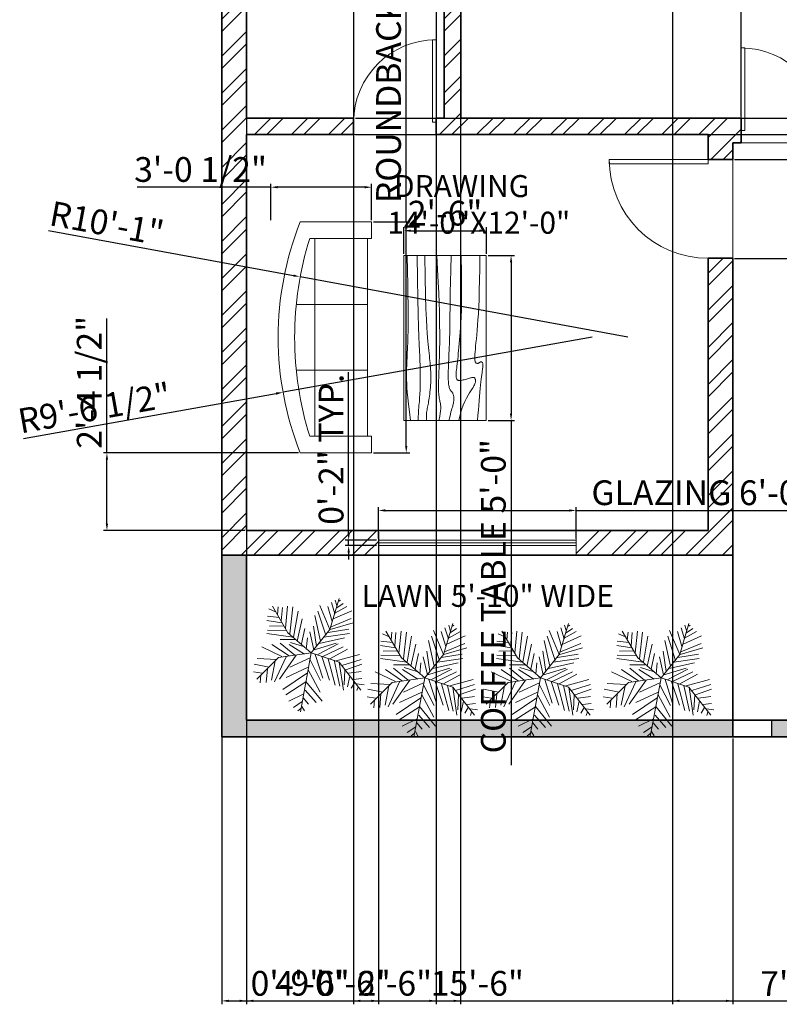
# Model space of a CAD drawing. Units: inches. Extents: x 177 to 1423, y 532 to 2503.
# Tile 1 of 5: x 177 to 453, y 539 to 897. Entities that reach past the tile are written whole.
import ezdxf

# ---------------------------------------------------------------- set-up
doc = ezdxf.new("R2010")
doc.units = ezdxf.units.IN
for name, color, linetype, lineweight in [('A-ANNO-DIMS', 2, 'Continuous', 18), ('A-AREA-IDEN', 7, 'Continuous', 18), ('A-DOOR', 4, 'Continuous', 18), ('A-FURN', 8, 'Continuous', 18), ('A-GLAZ', 244, 'Continuous', 18), ('A-SITE-GATE', 244, 'Continuous', 25), ('A-WALL', 7, 'Continuous', 35), ('A-WALL-PATT', 252, 'Continuous', 13), ('L-PLNT', 94, 'Continuous', 13)]:
    doc.layers.add(name, color=color, linetype=linetype, lineweight=lineweight)
doc.styles.get("Standard").update_dxf_attribs({"font": 'arial.ttf'})
doc.dimstyles.new('ISO-25', dxfattribs={"dimtxt": 9, "dimasz": 2.5, "dimexe": 1.25, "dimexo": 0.625, "dimtad": 1, "dimlunit": 3, "dimtxsty": 'Standard', "dimcen": 2.5, "dimadec": 0, "dimazin": 0, "dimtfac": 1, "dimtmove": 0, "dimatfit": 3, "dimfxl": 1, "dimarcsym": 0})

# ---------------------------------------------------------------- blocks, each defined once
blk = doc.blocks.new('*U2')
for p, q in [((0, 0), (0, -6)), ((40, 0), (40, -6))]:
    blk.add_line(p, q)
blk.add_lwpolyline([(0, 0), (0, 40), (1.75, 40), (1.75, 0)], close=True)
blk.add_arc((0, 0), 40, 0, 90)
blk = doc.blocks.new('*U4')
for p, q in [((-40, 0), (-40, 6)), ((0, 0), (0, 6))]:
    blk.add_line(p, q)
blk.add_lwpolyline([(0, 0), (0, -40), (-1.75, -40), (-1.75, 0)], close=True)
blk.add_arc((0, 0), 40, 180, 270)
blk = doc.blocks.new('*U11')
for p, q in [((-8.737, 47.138), (-17.069, 52.711)), ((-10.186, 53.64), (-13.084, 55.962)), ((0, 0), (-10.5, 57)), ((-9.099, 51.782), (-6.563, 55.962)), ((-7.65, 43.423), (-2.578, 49.46)), ((-5.839, 35.992), (4.667, 48.067)), ((-5.114, 28.097), (-24.676, 40.636)), ((-7.288, 39.707), (-21.778, 46.673)), ((-5.114, 27.632), (10.463, 46.673)), ((-48.585, 21.131), (-49.309, 29.026)), ((-43.513, 28.561), (-42.427, 15.558)), ((-3.665, 19.273), (-27.574, 35.527)), ((-2.941, 16.486), (8.652, 37.85)), ((16.259, 5.805), (23.142, 31.348)), ((22.055, 7.198), (27.489, 32.277)), ((27, 9), (48, 36)), ((27.127, 9.056), (31.112, 35.992)), ((31.836, 30.883), (32.561, 16.486)), ((35.096, 32.741), (37.27, 22.524)), ((38.719, 34.134), (41.979, 28.561)), ((43.791, 29.954), (51.036, 30.883)), ((44.153, 36.456), (45.239, 32.741)), ((-47.498, 19.737), (-55.83, 18.344)), ((-31.5, 4.5), (-52.5, 25.5)), ((-38.442, 26.239), (-34.819, 7.663)), ((-35.544, 28.097), (-24.314, 3.947)), ((-14.533, 2.09), (-30.834, 25.31)), ((-24.314, 23.917), (-2.941, 13.7)), ((-1.129, 6.734), (9.014, 26.704)), ((3.942, 1.625), (11.187, 24.381)), ((10.101, 3.483), (17.708, 26.239)), ((36.183, 19.737), (48.137, 17.88)), ((40.53, 25.775), (48.862, 24.846)), ((-40.615, 13.7), (-55.105, 10.913)), ((-20.691, 13.7), (-1.129, 4.876)), ((29.662, 12.307), (48.137, 6.269)), ((33.285, 16.486), (48.862, 10.913)), ((-33.37, 6.269), (-52.207, 5.34)), ((-28.299, 3.483), (-47.86, -5.805)), ((-21.416, 3.018), (-38.079, -8.128)), ((0, 0), (-31.5, 4.5)), ((-15.982, 2.09), (-30.11, -9.521)), ((0, 0), (-22.5, -19.5)), ((-6.563, 1.161), (-21.416, -8.128)), ((0, 0), (27, 9)), ((0, 0), (18, -22.5)), ((6.478, 1.625), (26.04, -8.592)), ((11.187, 3.483), (30.749, -5.805)), ((18.07, 5.805), (35.096, -3.483)), ((24.229, 7.663), (46.688, 1.625)), ((-6.563, -5.805), (-19.967, -9.985)), ((-9.461, -8.592), (-6.201, -23.453)), ((-4.752, -3.483), (-3.665, -14.629)), ((2.493, -3.019), (-1.491, -20.202)), ((1.769, -2.555), (24.229, -9.521)), ((5.029, -6.27), (2.131, -25.775)), ((7.565, -9.056), (32.198, -14.629)), ((-17.431, -15.094), (-42.789, -18.809)), ((-15.257, -12.772), (-30.11, -12.772)), ((-20.691, -18.345), (-17.793, -44.352)), ((-17.069, -15.094), (-12.721, -40.172)), ((-13.446, -11.378), (-8.737, -32.741)), ((9.014, -11.378), (3.58, -35.992)), ((14.085, -16.951), (6.478, -40.172)), ((12.274, -15.094), (36.907, -18.809)), ((-24.314, -21.596), (-42.427, -22.06)), ((-26.849, -26.24), (-40.253, -25.775)), ((-22.5, -19.5), (-37.5, -45)), ((-25.038, -23.918), (-22.865, -45.281)), ((18.07, -22.524), (8.289, -45.745)), ((16.259, -19.738), (36.183, -22.989)), ((18, -22.5), (27, -52.5)), ((18.433, -22.524), (40.53, -29.026)), ((19.157, -25.311), (38.719, -33.206)), ((-28.299, -29.026), (-42.789, -31.348)), ((-30.834, -34.135), (-42.427, -35.528)), ((-32.646, -36.921), (-31.921, -44.352)), ((-29.023, -30.884), (-27.936, -43.887)), ((20.244, -30.419), (15.897, -44.816)), ((22.78, -37.85), (19.519, -48.532)), ((21.331, -32.741), (39.081, -40.636)), ((-34.457, -39.708), (-40.978, -42.494)), ((22.78, -38.314), (34.372, -44.816)), ((24.591, -45.745), (23.142, -50.854)), ((24.591, -43.423), (30.749, -47.603)), ((26.764, -49.925), (28.213, -50.854))]:
    blk.add_line(p, q)
blk = doc.blocks.new('Sofa - Roundback 7 ft.')
for p, q in [((-12.00002, -32.4421), (-12.00003, -6.5971)), ((11.99997, -32.4421), (11.99998, -6.5971)), ((-36.000027, -34), (-36.000027, -11.4696)), ((-35.999844, -13.3819), (35.9998, -13.3819)), ((35.99998, -34), (35.99998, -11.4696)), ((-36.000027, -32.4421), (35.99998, -32.4421))]:
    blk.add_line(p, q)
for points in [[(-36.000027, -34), (-42.000027, -34), (-42.000027, -8)], [(41.99998, -8), (41.99998, -34), (35.99998, -34)]]:
    blk.add_lwpolyline(points)
for centre, radius, start, end in [((0, -114.25), 114.25, 68.43141, 111.5686), ((-0.00001, -127.1968), 121.1968, 72.72033, 107.2797)]:
    blk.add_arc(centre, radius, start, end)
blk = doc.blocks.new('Table - Rectangular Woodgrain 60 x 30 in.')
for p, q in [((0, 0), (0, -30)), ((60, 0), (0, 0)), ((60, -30), (60, 0)), ((0, -30), (60, -30))]:
    blk.add_line(p, q)
for points in [[(0, -2.4), (4.8155, -2.418), (9.0302, -2.4688), (12.709, -2.5477), (15.9167, -2.65), (18.7181, -2.7711), (21.1781, -2.9063), (23.3616, -3.0508), (25.3333, -3.2), (27.1477, -3.3495), (28.8172, -3.4958), (30.3437, -3.636), (31.7291, -3.7667), (32.9756, -3.8849), (34.0849, -3.9875), (35.059, -4.0714), (35.9, -4.1334), (36.6114, -4.1711), (37.2041, -4.1854), (37.6906, -4.1779), (38.0833, -4.15), (38.3948, -4.1034), (38.6375, -4.0396), (38.8239, -3.9602), (38.9666, -3.8667), (39.0764, -3.7608), (39.1573, -3.6448), (39.2116, -3.521), (39.2416, -3.3917), (39.2498, -3.2593), (39.2385, -3.1261), (39.21, -2.9944), (39.1666, -2.8667), (39.111, -2.7447), (39.0468, -2.6281), (38.978, -2.5163), (38.9083, -2.4083), (38.8418, -2.3035), (38.7823, -2.201), (38.7337, -2.1001), (38.7, -2), (38.6844, -1.9003), (38.6875, -1.8021), (38.7094, -1.707), (38.75, -1.6167), (38.8094, -1.5326), (38.8875, -1.4563), (38.9844, -1.3893), (39.1, -1.3333), (39.2351, -1.2896), (39.3937, -1.2583), (39.5804, -1.2396), (39.8, -1.2333), (40.057, -1.2396), (40.3562, -1.2583), (40.7023, -1.2896), (41.1, -1.3333), (41.5547, -1.3895), (42.0755, -1.4573), (42.6721, -1.5361), (43.3542, -1.625), (44.1316, -1.7233), (45.014, -1.8302), (46.0114, -1.9449), (47.1333, -2.0667), (48.3862, -2.1947), (49.7625, -2.3281), (51.2513, -2.4663), (52.8416, -2.6083), (54.5226, -2.7535), (56.2833, -2.9011), (58.1127, -3.0501), (60, -3.2)], [(0, -9.2), (6.5759, -9.0858), (11.9385, -9.0365), (16.2527, -9.0418), (19.6833, -9.0917), (22.3952, -9.1759), (24.5531, -9.2844), (26.322, -9.4069), (27.8666, -9.5333), (29.3241, -9.6553), (30.7203, -9.7719), (32.0532, -9.8837), (33.3208, -9.9917), (34.5213, -10.0965), (35.6526, -10.199), (36.7128, -10.2999), (37.7, -10.4), (38.6129, -10.4996), (39.4531, -10.5969), (40.223, -10.6895), (40.925, -10.775), (41.5613, -10.8512), (42.1344, -10.9156), (42.6465, -10.966), (43.1, -11), (43.4976, -11.0158), (43.8437, -11.0136), (44.143, -10.9942), (44.4, -10.9583), (44.6195, -10.9069), (44.8062, -10.8406), (44.9648, -10.7603), (45.1, -10.6667), (45.2155, -10.5598), (45.3114, -10.4365), (45.3871, -10.2929), (45.4416, -10.125), (45.4743, -9.929), (45.4844, -9.7011), (45.4709, -9.4371), (45.4333, -9.1333), (45.3716, -8.7883), (45.2896, -8.4104), (45.1919, -8.0107), (45.0833, -7.6), (44.9685, -7.1893), (44.8521, -6.7896), (44.7388, -6.4117), (44.6333, -6.0667), (44.54, -5.7628), (44.4614, -5.4979), (44.4001, -5.2675), (44.3583, -5.0667), (44.3384, -4.8909), (44.3427, -4.7354), (44.3736, -4.5956), (44.4333, -4.4667), (44.5236, -4.3453), (44.6427, -4.2333), (44.7884, -4.1339), (44.9583, -4.05), (45.1501, -3.9849), (45.3614, -3.9417), (45.59, -3.9234), (45.8333, -3.9333), (46.0915, -3.9749), (46.3734, -4.0531), (46.6906, -4.1736), (47.0542, -4.3417), (47.4756, -4.5629), (47.9661, -4.8427), (48.5372, -5.1866), (49.2, -5.6), (49.9676, -6.0844), (50.8594, -6.625), (51.8965, -7.2031), (53.1, -7.8), (54.491, -8.3969), (56.0906, -8.975), (57.9199, -9.5156), (60, -10)], [(0, -12.8), (5.1847, -12.9322), (9.6213, -13.0323), (13.3963, -13.1059), (16.5958, -13.1583), (19.3063, -13.1952), (21.614, -13.2219), (23.6054, -13.2439), (25.3666, -13.2667), (26.9728, -13.2947), (28.4531, -13.3281), (29.8256, -13.3663), (31.1083, -13.4083), (32.3191, -13.4535), (33.476, -13.501), (34.597, -13.5501), (35.7, -13.6), (36.7984, -13.6497), (37.8875, -13.6979), (38.9578, -13.743), (40, -13.7833), (41.0047, -13.8174), (41.9625, -13.8438), (42.864, -13.8607), (43.7, -13.8667), (44.4631, -13.8604), (45.1552, -13.8417), (45.7801, -13.8104), (46.3416, -13.7667), (46.8439, -13.7104), (47.2906, -13.6417), (47.6858, -13.5604), (48.0333, -13.4667), (48.3375, -13.3608), (48.6042, -13.2448), (48.8396, -13.121), (49.05, -12.9917), (49.2417, -12.8593), (49.4208, -12.7261), (49.5937, -12.5944), (49.7667, -12.4667), (49.9452, -12.3451), (50.1323, -12.2313), (50.3303, -12.1268), (50.5416, -12.0333), (50.7686, -11.9524), (51.0135, -11.8854), (51.2788, -11.8341), (51.5666, -11.8), (51.8785, -11.7843), (52.2116, -11.7865), (52.562, -11.8059), (52.926, -11.8417), (53.2998, -11.8931), (53.6795, -11.9594), (54.0614, -12.0397), (54.4416, -12.1333), (54.8223, -12.2401), (55.2293, -12.3625), (55.6942, -12.5037), (56.2489, -12.6667), (56.9251, -12.8547), (57.7545, -13.0708), (58.7689, -13.3182), (60, -13.6)], [(0, -18), (5.124, -17.7273), (9.6609, -17.5057), (13.6705, -17.3303), (17.2125, -17.1958), (20.3467, -17.0973), (23.1328, -17.0297), (25.6307, -16.9878), (27.9, -16.9667), (29.9928, -16.9617), (31.9302, -16.9703), (33.7254, -16.9907), (35.3917, -17.0208), (36.9423, -17.0588), (38.3906, -17.1026), (39.7499, -17.1503), (41.0333, -17.2), (42.2519, -17.2496), (43.4073, -17.2969), (44.4986, -17.3395), (45.525, -17.375), (46.4858, -17.4012), (47.3802, -17.4156), (48.2074, -17.416), (48.9667, -17.4), (49.6583, -17.3662), (50.2872, -17.3167), (50.8595, -17.2547), (51.3812, -17.1833), (51.8584, -17.1057), (52.2971, -17.025), (52.7034, -16.9443), (53.0833, -16.8667), (53.443, -16.7951), (53.789, -16.7313), (54.128, -16.6768), (54.4666, -16.6334), (54.8115, -16.6024), (55.1693, -16.5854), (55.5465, -16.5841), (55.95, -16.6), (56.3828, -16.6337), (56.8346, -16.6823), (57.2915, -16.7418), (57.7396, -16.8084), (58.165, -16.878), (58.5539, -16.9469), (58.8924, -17.0111), (59.1666, -17.0667), (59.3679, -17.1107), (59.5078, -17.1438), (59.6032, -17.1675), (59.6708, -17.1833), (59.7275, -17.193), (59.7901, -17.1979), (59.8753, -17.1998), (60, -17.2)], [(0, -22.4), (8.0098, -22.2501), (14.4094, -22.1011), (19.4168, -21.9535), (23.25, -21.8083), (26.1269, -21.6663), (28.2656, -21.5281), (29.884, -21.3947), (31.2, -21.2667), (32.3967, -21.1448), (33.5172, -21.0292), (34.5697, -20.9198), (35.5625, -20.8167), (36.5037, -20.7198), (37.4015, -20.6292), (38.2642, -20.5448), (39.1, -20.4667), (39.9164, -20.3951), (40.7187, -20.3313), (41.5117, -20.2768), (42.3, -20.2333), (43.0883, -20.2024), (43.8812, -20.1854), (44.6836, -20.1841), (45.5, -20.2), (46.3328, -20.234), (47.1747, -20.2844), (48.0163, -20.3488), (48.8479, -20.425), (49.66, -20.5106), (50.4429, -20.6031), (51.1872, -20.7004), (51.8833, -20.8), (52.5246, -20.8999), (53.1166, -20.9995), (53.6681, -21.0983), (54.1875, -21.1958), (54.6834, -21.2919), (55.1646, -21.3859), (55.6394, -21.4777), (56.1167, -21.5667), (56.6028, -21.6515), (57.0961, -21.7266), (57.5929, -21.7852), (58.0896, -21.8208), (58.5823, -21.8268), (59.0674, -21.7964), (59.5412, -21.723), (60, -21.6)], [(0, -25.2), (8.6355, -25.0504), (15.7026, -24.9031), (21.4049, -24.7606), (25.9458, -24.625), (29.529, -24.4988), (32.3578, -24.3844), (34.6359, -24.284), (36.5667, -24.2), (38.3213, -24.1341), (39.9417, -24.0854), (41.437, -24.0523), (42.8167, -24.0333), (44.0901, -24.0268), (45.2667, -24.0313), (46.3557, -24.0451), (47.3667, -24.0667), (48.309, -24.0947), (49.1928, -24.1287), (50.0284, -24.168), (50.826, -24.2125), (51.5959, -24.2617), (52.3483, -24.3151), (53.0935, -24.3725), (53.8417, -24.4334), (54.6009, -24.497), (55.3699, -24.561), (56.1454, -24.6226), (56.9239, -24.6792), (57.7021, -24.7279), (58.4764, -24.7662), (59.2435, -24.7911), (60, -24.8)], [(0, -28.8), (5.6867, -28.6681), (10.45, -28.5698), (14.407, -28.5012), (17.675, -28.4584), (20.3711, -28.4374), (22.6125, -28.4344), (24.5164, -28.4455), (26.2, -28.4667), (27.762, -28.4947), (29.2276, -28.5281), (30.6033, -28.5663), (31.8958, -28.6084), (33.1118, -28.6535), (34.2578, -28.7011), (35.3405, -28.7501), (36.3666, -28.8), (37.3443, -28.8497), (38.288, -28.8974), (39.2137, -28.9412), (40.1375, -28.9792), (41.0753, -29.0093), (42.0432, -29.0297), (43.0572, -29.0384), (44.1333, -29.0333), (45.2936, -29.0114), (46.5843, -28.9641), (48.0579, -28.8816), (49.7666, -28.7542), (51.7629, -28.5721), (54.0989, -28.3255), (56.8272, -28.0048), (60, -27.6)]]:
    blk.add_lwpolyline(points)
blk = doc.blocks.new('WIN-GLAZING-72IN')
for p, q in [((72, 2), (0, 2)), ((72, 1), (0, 1)), ((72, 0), (0, 0))]:
    blk.add_line(p, q)
blk = doc.blocks.new('*D24')
at = {"layer": 'A-ANNO-DIMS', "color": 0, "lineweight": -2, "transparency": 16777216}
for p, q in [((307.55, 708.28), (307.55, 719.7)), ((310.05, 718.45), (377.05, 718.45)), ((379.55, 708.28), (379.55, 719.7)), ((379.55, 718.45), (496.7, 718.45))]:
    blk.add_line(p, q, dxfattribs=at)
at = {"layer": 'A-ANNO-DIMS', "color": 0, "transparency": 16777216}
for points in [[(310.05, 718.87), (310.05, 718.04), (307.55, 718.45)], [(377.05, 718.87), (377.05, 718.04), (379.55, 718.45)]]:
    blk.add_solid(points, dxfattribs=at)
at = {"layer": 'Defpoints', "color": 0, "transparency": 16777216}
for p in [(379.55, 718.45), (307.55, 707.65), (379.55, 707.65)]:
    blk.add_point(p, dxfattribs=at)
at = {"layer": 'A-ANNO-DIMS', "color": 0, "transparency": 16777216, "insert": (439.37, 723.73), "char_height": 9, "attachment_point": 5}
blk.add_mtext('GLAZING 6\'-0" TYP.', dxfattribs=at)
blk = doc.blocks.new('*D25')
at = {"layer": 'A-ANNO-DIMS', "color": 0, "lineweight": -2, "transparency": 16777216}
for p, q in [((296.75, 710.15), (296.75, 768.76)), ((306.93, 707.65), (295.5, 707.65)), ((306.93, 705.65), (295.5, 705.65)), ((296.75, 705.65), (296.75, 707.65)), ((296.75, 703.15), (296.75, 700.65))]:
    blk.add_line(p, q, dxfattribs=at)
at = {"layer": 'A-ANNO-DIMS', "color": 0, "transparency": 16777216}
for points in [[(296.33, 710.15), (297.17, 710.15), (296.75, 707.65)], [(296.33, 703.15), (297.17, 703.15), (296.75, 705.65)]]:
    blk.add_solid(points, dxfattribs=at)
at = {"layer": 'Defpoints', "color": 0, "transparency": 16777216}
for p in [(296.75, 707.65), (307.55, 707.65), (307.55, 705.65)]:
    blk.add_point(p, dxfattribs=at)
at = {"layer": 'A-ANNO-DIMS', "color": 0, "transparency": 16777216, "insert": (291.53, 740.71), "char_height": 9, "attachment_point": 5, "rotation": 90}
blk.add_mtext('0\'-2" TYP.', dxfattribs=at)
blk = doc.blocks.new('*D30')
at = {"layer": 'A-ANNO-DIMS', "color": 0, "lineweight": -2, "transparency": 16777216}
for p, q in [((347.46, 811.2), (357.09, 811.2)), ((355.84, 808.7), (355.84, 753.7)), ((347.46, 751.2), (357.09, 751.2)), ((355.84, 751.2), (355.84, 625.82))]:
    blk.add_line(p, q, dxfattribs=at)
at = {"layer": 'A-ANNO-DIMS', "color": 0, "transparency": 16777216}
for points in [[(355.42, 808.7), (356.25, 808.7), (355.84, 811.2)], [(355.42, 753.7), (356.25, 753.7), (355.84, 751.2)]]:
    blk.add_solid(points, dxfattribs=at)
at = {"layer": 'Defpoints', "color": 0, "transparency": 16777216}
for p in [(346.84, 811.2), (346.84, 751.2), (355.84, 751.2)]:
    blk.add_point(p, dxfattribs=at)
at = {"layer": 'A-ANNO-DIMS', "color": 0, "transparency": 16777216, "insert": (350.55, 687.26), "char_height": 9, "attachment_point": 5, "rotation": 90}
blk.add_mtext('COFFEE TABLE 5\'-0"', dxfattribs=at)
blk = doc.blocks.new('*D31')
at = {"layer": 'A-ANNO-DIMS', "color": 0, "lineweight": -2, "transparency": 16777216}
for p, q in [((316.84, 811.82), (316.84, 821.45)), ((319.34, 820.2), (344.34, 820.2)), ((346.84, 811.82), (346.84, 821.45))]:
    blk.add_line(p, q, dxfattribs=at)
at = {"layer": 'A-ANNO-DIMS', "color": 0, "transparency": 16777216}
for points in [[(319.34, 820.61), (319.34, 819.78), (316.84, 820.2)], [(344.34, 820.61), (344.34, 819.78), (346.84, 820.2)]]:
    blk.add_solid(points, dxfattribs=at)
at = {"layer": 'Defpoints', "color": 0, "transparency": 16777216}
for p in [(346.84, 820.2), (316.84, 811.2), (346.84, 811.2)]:
    blk.add_point(p, dxfattribs=at)
at = {"layer": 'A-ANNO-DIMS', "color": 0, "transparency": 16777216, "insert": (331.84, 825.42), "char_height": 9, "attachment_point": 5}
blk.add_mtext('2\'-6"', dxfattribs=at)
blk = doc.blocks.new('*D32')
at = {"layer": 'A-ANNO-DIMS', "color": 0, "lineweight": -2, "transparency": 16777216}
for p, q in [((317.7, 823.42), (317.7, 972.18)), ((305.73, 823.42), (318.95, 823.42)), ((317.7, 741.92), (317.7, 820.92)), ((305.73, 739.42), (318.95, 739.42))]:
    blk.add_line(p, q, dxfattribs=at)
at = {"layer": 'A-ANNO-DIMS', "color": 0, "transparency": 16777216}
for points in [[(317.29, 820.92), (318.12, 820.92), (317.7, 823.42)], [(317.29, 741.92), (318.12, 741.92), (317.7, 739.42)]]:
    blk.add_solid(points, dxfattribs=at)
at = {"layer": 'Defpoints', "color": 0, "transparency": 16777216}
for p in [(305.1, 823.42), (317.7, 823.42), (305.1, 739.42)]:
    blk.add_point(p, dxfattribs=at)
at = {"layer": 'A-ANNO-DIMS', "color": 0, "transparency": 16777216, "insert": (312.42, 899.05), "char_height": 9, "attachment_point": 5, "rotation": 90}
blk.add_mtext('ROUNDBACK SOFA 7\'-0"', dxfattribs=at)
blk = doc.blocks.new('*D33')
at = {"layer": 'A-ANNO-DIMS', "color": 0, "lineweight": -2, "transparency": 16777216}
for p, q in [((268.44, 836.02), (219.8, 836.02)), ((268.44, 824.04), (268.44, 837.27)), ((302.6, 836.02), (270.94, 836.02)), ((305.1, 824.04), (305.1, 837.27))]:
    blk.add_line(p, q, dxfattribs=at)
at = {"layer": 'A-ANNO-DIMS', "color": 0, "transparency": 16777216}
for points in [[(270.94, 836.44), (270.94, 835.6), (268.44, 836.02)], [(302.6, 836.44), (302.6, 835.6), (305.1, 836.02)]]:
    blk.add_solid(points, dxfattribs=at)
at = {"layer": 'Defpoints', "color": 0, "transparency": 16777216}
for p in [(268.44, 836.02), (268.44, 823.42), (305.1, 823.42)]:
    blk.add_point(p, dxfattribs=at)
at = {"layer": 'A-ANNO-DIMS', "color": 0, "transparency": 16777216, "insert": (242.87, 841.3), "char_height": 9, "attachment_point": 5}
blk.add_mtext('3\'-0 1/2"', dxfattribs=at)
blk = doc.blocks.new('*D34')
at = {"layer": 'A-ANNO-DIMS', "color": 0, "lineweight": -2, "transparency": 16777216}
for p, q in [((250.55, 635.53), (250.55, 538.84)), ((436.55, 635.53), (436.55, 538.84)), ((253.05, 540.09), (434.05, 540.09))]:
    blk.add_line(p, q, dxfattribs=at)
at = {"layer": 'A-ANNO-DIMS', "color": 0, "transparency": 16777216}
for points in [[(253.05, 540.51), (253.05, 539.68), (250.55, 540.09)], [(434.05, 540.51), (434.05, 539.68), (436.55, 540.09)]]:
    blk.add_solid(points, dxfattribs=at)
at = {"layer": 'Defpoints', "color": 0, "transparency": 16777216}
for p in [(250.55, 636.15), (436.55, 636.15), (436.55, 540.09)]:
    blk.add_point(p, dxfattribs=at)
at = {"layer": 'A-ANNO-DIMS', "color": 0, "transparency": 16777216, "insert": (343.55, 545.31), "char_height": 9, "attachment_point": 5}
blk.add_mtext('15\'-6"', dxfattribs=at)
blk = doc.blocks.new('*D40')
at = {"layer": 'A-ANNO-DIMS', "color": 0, "lineweight": -2, "transparency": 16777216}
for p, q in [((414.55, 1172.53), (414.55, 538.84)), ((505.55, 1172.53), (505.55, 538.84)), ((417.05, 540.09), (503.05, 540.09))]:
    blk.add_line(p, q, dxfattribs=at)
at = {"layer": 'A-ANNO-DIMS', "color": 0, "transparency": 16777216}
for points in [[(417.05, 540.51), (417.05, 539.68), (414.55, 540.09)], [(503.05, 540.51), (503.05, 539.68), (505.55, 540.09)]]:
    blk.add_solid(points, dxfattribs=at)
at = {"layer": 'Defpoints', "color": 0, "transparency": 16777216}
for p in [(414.55, 1173.15), (505.55, 1173.15), (505.55, 540.09)]:
    blk.add_point(p, dxfattribs=at)
at = {"layer": 'A-ANNO-DIMS', "color": 0, "transparency": 16777216, "insert": (460.05, 545.22), "char_height": 9, "attachment_point": 5}
blk.add_mtext('7\'-7"', dxfattribs=at)
blk = doc.blocks.new('*D41')
at = {"layer": 'A-ANNO-DIMS', "color": 0, "lineweight": -2, "transparency": 16777216}
for p, q in [((439.55, 861.78), (439.55, 1447.15)), ((499.55, 861.78), (499.55, 1447.15)), ((442.05, 1445.9), (497.05, 1445.9))]:
    blk.add_line(p, q, dxfattribs=at)
at = {"layer": 'A-ANNO-DIMS', "color": 0, "transparency": 16777216}
for points in [[(442.05, 1446.32), (442.05, 1445.49), (439.55, 1445.9)], [(497.05, 1446.32), (497.05, 1445.49), (499.55, 1445.9)]]:
    blk.add_solid(points, dxfattribs=at)
at = {"layer": 'Defpoints', "color": 0, "transparency": 16777216}
for p in [(499.55, 1445.9), (439.55, 861.15), (499.55, 861.15)]:
    blk.add_point(p, dxfattribs=at)
at = {"layer": 'A-ANNO-DIMS', "color": 0, "transparency": 16777216, "insert": (469.55, 1451.12), "char_height": 9, "attachment_point": 5}
blk.add_mtext('5\'-0"', dxfattribs=at)
blk = doc.blocks.new('*D42')
at = {"layer": 'A-ANNO-DIMS', "color": 0, "lineweight": -2, "transparency": 16777216}
for p, q in [((259.55, 710.53), (259.55, 538.84)), ((250.55, 701.53), (250.55, 538.84)), ((253.05, 540.09), (257.05, 540.09)), ((259.55, 540.09), (287.22, 540.09))]:
    blk.add_line(p, q, dxfattribs=at)
at = {"layer": 'A-ANNO-DIMS', "color": 0, "transparency": 16777216}
for points in [[(253.05, 540.51), (253.05, 539.68), (250.55, 540.09)], [(257.05, 540.51), (257.05, 539.68), (259.55, 540.09)]]:
    blk.add_solid(points, dxfattribs=at)
at = {"layer": 'Defpoints', "color": 0, "transparency": 16777216}
for p in [(259.55, 711.15), (250.55, 702.15), (259.55, 540.09)]:
    blk.add_point(p, dxfattribs=at)
at = {"layer": 'A-ANNO-DIMS', "color": 0, "transparency": 16777216, "insert": (274.64, 545.31), "char_height": 9, "attachment_point": 5}
blk.add_mtext('0\'-9"', dxfattribs=at)
blk = doc.blocks.new('*D43')
at = {"layer": 'A-ANNO-DIMS', "color": 0, "lineweight": -2, "transparency": 16777216}
for p, q in [((766.3, 863.65), (766.3, 891.33)), ((299.18, 861.15), (767.55, 861.15)), ((766.3, 855.15), (766.3, 861.15)), ((299.18, 855.15), (767.55, 855.15)), ((766.3, 852.65), (766.3, 850.15))]:
    blk.add_line(p, q, dxfattribs=at)
at = {"layer": 'A-ANNO-DIMS', "color": 0, "transparency": 16777216}
for points in [[(765.88, 863.65), (766.72, 863.65), (766.3, 861.15)], [(765.88, 852.65), (766.72, 852.65), (766.3, 855.15)]]:
    blk.add_solid(points, dxfattribs=at)
at = {"layer": 'Defpoints', "color": 0, "transparency": 16777216}
for p in [(298.55, 861.15), (766.3, 861.15), (298.55, 855.15)]:
    blk.add_point(p, dxfattribs=at)
at = {"layer": 'A-ANNO-DIMS', "color": 0, "transparency": 16777216, "insert": (761.08, 878.74), "char_height": 9, "attachment_point": 5, "rotation": 90}
blk.add_mtext('0\'-6"', dxfattribs=at)
blk = doc.blocks.new('*D44')
at = {"layer": 'A-ANNO-DIMS', "color": 0, "lineweight": -2, "transparency": 16777216}
for p, q in [((437.18, 846.15), (767.55, 846.15)), ((766.3, 812.65), (766.3, 843.65)), ((437.18, 810.15), (767.55, 810.15))]:
    blk.add_line(p, q, dxfattribs=at)
at = {"layer": 'A-ANNO-DIMS', "color": 0, "transparency": 16777216}
for points in [[(765.88, 843.65), (766.72, 843.65), (766.3, 846.15)], [(765.88, 812.65), (766.72, 812.65), (766.3, 810.15)]]:
    blk.add_solid(points, dxfattribs=at)
at = {"layer": 'Defpoints', "color": 0, "transparency": 16777216}
for p in [(436.55, 846.15), (766.3, 846.15), (436.55, 810.15)]:
    blk.add_point(p, dxfattribs=at)
at = {"layer": 'A-ANNO-DIMS', "color": 0, "transparency": 16777216, "insert": (761.08, 828.15), "char_height": 9, "attachment_point": 5, "rotation": 90}
blk.add_mtext('3\'-0"', dxfattribs=at)
blk = doc.blocks.new('*D45')
at = {"layer": 'A-ANNO-DIMS', "color": 0, "lineweight": -2, "transparency": 16777216}
for p, q in [((259.55, 710.53), (259.55, 538.84)), ((307.55, 710.53), (307.55, 538.84)), ((262.05, 540.09), (305.05, 540.09))]:
    blk.add_line(p, q, dxfattribs=at)
at = {"layer": 'A-ANNO-DIMS', "color": 0, "transparency": 16777216}
for points in [[(262.05, 540.51), (262.05, 539.68), (259.55, 540.09)], [(305.05, 540.51), (305.05, 539.68), (307.55, 540.09)]]:
    blk.add_solid(points, dxfattribs=at)
at = {"layer": 'Defpoints', "color": 0, "transparency": 16777216}
for p in [(259.55, 711.15), (307.55, 711.15), (307.55, 540.09)]:
    blk.add_point(p, dxfattribs=at)
at = {"layer": 'A-ANNO-DIMS', "color": 0, "transparency": 16777216, "insert": (283.55, 545.31), "char_height": 9, "attachment_point": 5}
blk.add_mtext('4\'-0"', dxfattribs=at)
blk = doc.blocks.new('*D46')
at = {"layer": 'A-ANNO-DIMS', "color": 0, "lineweight": -2, "transparency": 16777216}
for p, q in [((208.8, 739.42), (208.8, 788.22)), ((278.48, 739.42), (207.55, 739.42)), ((208.8, 713.65), (208.8, 736.92)), ((258.93, 711.15), (207.55, 711.15))]:
    blk.add_line(p, q, dxfattribs=at)
at = {"layer": 'A-ANNO-DIMS', "color": 0, "transparency": 16777216}
for points in [[(208.38, 736.92), (209.22, 736.92), (208.8, 739.42)], [(208.38, 713.65), (209.22, 713.65), (208.8, 711.15)]]:
    blk.add_solid(points, dxfattribs=at)
at = {"layer": 'Defpoints', "color": 0, "transparency": 16777216}
for p in [(208.8, 739.42), (279.1, 739.42), (259.55, 711.15)]:
    blk.add_point(p, dxfattribs=at)
at = {"layer": 'A-ANNO-DIMS', "color": 0, "transparency": 16777216, "insert": (203.52, 765.07), "char_height": 9, "attachment_point": 5, "rotation": 90}
blk.add_mtext('2\'-4 1/2"', dxfattribs=at)
blk = doc.blocks.new('*D49')
at = {"layer": 'A-ANNO-DIMS', "color": 0, "lineweight": -2, "transparency": 16777216}
for p, q in [((259.55, 1052.53), (259.55, 538.84)), ((337.49, 1052.53), (337.49, 538.84)), ((262.05, 540.09), (334.99, 540.09))]:
    blk.add_line(p, q, dxfattribs=at)
at = {"layer": 'A-ANNO-DIMS', "color": 0, "transparency": 16777216}
for points in [[(262.05, 540.51), (262.05, 539.68), (259.55, 540.09)], [(334.99, 540.51), (334.99, 539.68), (337.49, 540.09)]]:
    blk.add_solid(points, dxfattribs=at)
at = {"layer": 'Defpoints', "color": 0, "transparency": 16777216}
for p in [(259.55, 1053.15), (337.49, 1053.15), (337.49, 540.09)]:
    blk.add_point(p, dxfattribs=at)
at = {"layer": 'A-ANNO-DIMS', "color": 0, "transparency": 16777216, "insert": (298.52, 545.31), "char_height": 9, "attachment_point": 5}
blk.add_mtext('6\'-6"', dxfattribs=at)
blk = doc.blocks.new('*D56')
at = {"layer": 'A-ANNO-DIMS', "color": 0, "lineweight": -2, "transparency": 16777216}
for p, q in [((298.55, 1259.53), (298.55, 538.84)), ((328.55, 1259.53), (328.55, 538.84)), ((301.05, 540.09), (326.05, 540.09))]:
    blk.add_line(p, q, dxfattribs=at)
at = {"layer": 'A-ANNO-DIMS', "color": 0, "transparency": 16777216}
for points in [[(301.05, 540.51), (301.05, 539.68), (298.55, 540.09)], [(326.05, 540.51), (326.05, 539.68), (328.55, 540.09)]]:
    blk.add_solid(points, dxfattribs=at)
at = {"layer": 'Defpoints', "color": 0, "transparency": 16777216}
for p in [(298.55, 1260.15), (328.55, 1260.15), (328.55, 540.09)]:
    blk.add_point(p, dxfattribs=at)
at = {"layer": 'A-ANNO-DIMS', "color": 0, "transparency": 16777216, "insert": (313.55, 545.31), "char_height": 9, "attachment_point": 5}
blk.add_mtext('2\'-6"', dxfattribs=at)
blk = doc.blocks.new('*D58')
at = {"layer": 'A-ANNO-DIMS', "color": 0, "lineweight": -2, "transparency": 16777216}
for p, q in [((187.56, 820.32), (276.66, 803.87)), ((398.3, 781.42), (279.12, 803.42))]:
    blk.add_line(p, q, dxfattribs=at)
at = {"layer": 'A-ANNO-DIMS', "color": 0, "transparency": 16777216}
blk.add_solid([(276.73, 804.28), (276.58, 803.46), (279.12, 803.42)], dxfattribs=at)
at = {"layer": 'Defpoints', "color": 0, "transparency": 16777216}
for p in [(279.12, 803.42), (398.3, 781.42)]:
    blk.add_point(p, dxfattribs=at)
at = {"layer": 'A-ANNO-DIMS', "color": 0, "transparency": 16777216, "insert": (208.55, 821.75), "char_height": 9, "attachment_point": 5, "rotation": 349.5409}
blk.add_mtext('R10\'-1"', dxfattribs=at)
blk = doc.blocks.new('*D59')
at = {"layer": 'A-ANNO-DIMS', "color": 0, "lineweight": -2, "transparency": 16777216}
for p, q in [((385.35, 781.42), (272.87, 761.42)), ((178.42, 744.62), (270.41, 760.98))]:
    blk.add_line(p, q, dxfattribs=at)
at = {"layer": 'A-ANNO-DIMS', "color": 0, "transparency": 16777216}
blk.add_solid([(270.33, 761.39), (270.48, 760.57), (272.87, 761.42)], dxfattribs=at)
at = {"layer": 'Defpoints', "color": 0, "transparency": 16777216}
for p in [(385.35, 781.42), (272.87, 761.42)]:
    blk.add_point(p, dxfattribs=at)
at = {"layer": 'A-ANNO-DIMS', "color": 0, "transparency": 16777216, "insert": (204.45, 754.61), "char_height": 9, "attachment_point": 5, "rotation": 10.0835}
blk.add_mtext('R9\'-6 1/2"', dxfattribs=at)

msp = doc.modelspace()

# ---------------------------------------------------------------- hatches: boundary and pattern name
at = {"layer": 'A-WALL-PATT'}
h = msp.add_hatch(dxfattribs=at)
h.set_pattern_fill('ANSI32', color=256)
h.paths.add_polyline_path([(436.55, 810.154), (427.55, 810.154), (427.55, 711.154), (379.55, 711.154), (379.55, 702.154), (436.55, 702.154)])
h.paths.add_polyline_path([(337.55, 963.154), (331.55, 963.154), (331.55, 951.154), (319.738, 951.154), (319.738, 945.154), (331.55, 945.154), (331.55, 861.154), (328.55, 861.154), (328.55, 855.154), (427.55, 855.154), (427.55, 846.154), (436.55, 846.154), (436.55, 852.154), (439.55, 852.154), (439.55, 861.154), (337.55, 861.154)], flags=17)
h.paths.add_polyline_path([(682.55, 1011.154), (643.55, 1011.154), (643.55, 1095.154), (701.063, 1095.154), (701.063, 1101.154), (700.55, 1101.154), (700.55, 1143.154), (691.55, 1143.154), (691.55, 1101.154), (511.55, 1101.154), (511.55, 1104.154), (505.55, 1104.154), (505.55, 1068.154), (511.55, 1068.154), (511.55, 1095.154), (637.55, 1095.154), (637.55, 1011.154), (511.55, 1011.154), (511.55, 1038.154), (505.55, 1038.154), (505.55, 1005.154), (541.55, 1005.154), (541.55, 1002.154), (547.55, 1002.154), (547.55, 1005.154), (682.55, 1005.154)], flags=17)
h.paths.add_polyline_path([(547.55, 966.154), (541.55, 966.154), (541.55, 861.154), (499.55, 861.154), (499.55, 852.154), (595.55, 852.154), (595.55, 861.154), (547.55, 861.154)], flags=17)
h.paths.add_polyline_path([(724.55, 1353.154), (337.55, 1353.154), (250.55, 1353.154), (250.55, 702.154), (307.55, 702.154), (307.55, 711.154), (259.55, 711.154), (259.55, 855.154), (298.55, 855.154), (298.55, 861.154), (259.55, 861.154), (259.55, 945.154), (298.738, 945.154), (298.738, 951.154), (259.55, 951.154), (259.55, 1047.154), (331.55, 1047.154), (331.55, 1035.154), (337.55, 1035.154), (337.55, 1047.154), (414.55, 1047.154), (414.55, 1056.154), (408.55, 1056.154), (408.55, 1053.154), (259.55, 1053.154), (259.55, 1173.154), (408.55, 1173.154), (408.55, 1092.154), (414.55, 1092.154), (414.55, 1173.154), (466.55, 1173.154), (466.55, 1179.154), (337.55, 1179.154), (337.55, 1194.154), (331.55, 1194.154), (331.55, 1179.154), (259.55, 1179.154), (259.55, 1194.154), (259.55, 1254.154), (298.55, 1254.154), (298.55, 1258.654), (298.55, 1260.154), (259.55, 1260.154), (259.55, 1344.154), (331.55, 1344.154), (331.55, 1346.691), (337.55, 1346.691), (337.55, 1347.154), (637.55, 1347.154), (637.55, 1346.676), (643.55, 1346.676), (643.55, 1344.154), (715.55, 1344.154), (715.55, 1263.154), (643.55, 1263.154), (643.55, 1266.154), (642.05, 1266.154), (637.55, 1266.154), (637.55, 1263.154), (610.55, 1263.154), (610.55, 1257.154), (691.55, 1257.154), (691.55, 1215.154), (700.55, 1215.154), (700.55, 1257.154), (718.55, 1257.154), (718.55, 1101.154), (715.137, 1101.154), (715.137, 1095.154), (715.55, 1095.154), (715.55, 1011.154), (712.55, 1011.154), (712.55, 1009.654), (712.55, 1005.154), (715.55, 1005.154), (715.55, 861.154), (667.55, 861.154), (667.55, 852.154), (724.55, 852.154)])
h.paths.add_polyline_path([(571.243, 1332.154), (457.55, 1332.154), (457.55, 1323.154), (505.55, 1323.154), (505.55, 1179.154), (502.55, 1179.154), (502.55, 1178.554), (502.55, 1173.154), (505.55, 1173.154), (505.55, 1140.154), (510.95, 1140.154), (511.55, 1140.154), (511.55, 1257.154), (574.55, 1257.154), (574.55, 1263.154), (511.55, 1263.154), (511.55, 1323.154), (571.243, 1323.154)], flags=17)
h.paths.add_polyline_path([(385.55, 1332.154), (337.55, 1332.154), (337.55, 1332.617), (331.55, 1332.617), (331.55, 1260.154), (328.55, 1260.154), (328.55, 1254.154), (337.55, 1254.154), (337.55, 1323.154), (385.55, 1323.154)], flags=17)
h.paths.add_polyline_path([(643.55, 1332.601), (637.55, 1332.601), (637.55, 1332.154), (607.243, 1332.154), (607.243, 1323.154), (637.55, 1323.154), (637.55, 1296.154), (642.05, 1296.154), (643.55, 1296.154)], flags=17)
h = msp.add_hatch(color=256, dxfattribs=at)
h.dxf.hatch_style = 1
h.paths.add_polyline_path([(462.585, 642.154), (450.585, 642.154), (450.585, 636.154), (462.585, 636.154)])
h.paths.add_polyline_path([(640.1, 642.154), (628.1, 642.154), (628.1, 636.154), (640.1, 636.154)])
h.paths.add_polyline_path([(724.55, 852.154), (715.55, 852.154), (715.55, 642.154), (661.3, 642.154), (661.3, 636.154), (724.55, 636.154)])
h.paths.add_polyline_path([(259.55, 702.154), (250.55, 702.154), (250.55, 636.154), (436.55, 636.154), (436.55, 642.154), (259.55, 642.154)])

# ---------------------------------------------------------------- linework, layer by layer
at = {"layer": 'A-DOOR'}
for p, q in [((298.55, 855.154), (328.55, 855.154)), ((439.55, 852.154), (499.55, 852.154)), ((436.55, 846.154), (436.55, 810.154))]:
    msp.add_line(p, q, dxfattribs=at)
at = {"layer": 'A-GLAZ'}
msp.add_lwpolyline([(307.55, 711.154), (379.55, 711.154), (379.55, 702.154), (307.55, 702.154)], close=True, dxfattribs=at)
at = {"layer": 'A-SITE-GATE'}
msp.add_line((450.585, 642.154), (450.585, 636.154), dxfattribs=at)
at = {"layer": 'A-WALL'}
for p, q in [((250.55, 1353.154), (250.55, 636.154)), ((337.55, 1047.154), (337.55, 861.154)), ((259.55, 945.154), (259.55, 861.154)), ((331.55, 945.154), (331.55, 861.154)), ((259.55, 861.154), (298.55, 861.154)), ((298.55, 861.154), (298.55, 855.154)), ((328.55, 861.154), (328.55, 855.154)), ((328.55, 861.154), (331.55, 861.154)), ((337.55, 861.154), (439.55, 861.154)), ((439.55, 852.154), (439.55, 861.154)), ((259.55, 855.154), (298.55, 855.154)), ((259.55, 855.154), (259.55, 711.154)), ((328.55, 855.154), (427.55, 855.154)), ((427.55, 855.154), (427.55, 846.154)), ((436.55, 852.154), (439.55, 852.154)), ((436.55, 852.154), (436.55, 846.154)), ((436.55, 846.154), (427.55, 846.154)), ((436.55, 810.154), (427.55, 810.154)), ((427.55, 810.154), (427.55, 711.154)), ((436.55, 810.154), (436.55, 636.154)), ((259.55, 711.154), (427.55, 711.154)), ((250.55, 702.154), (436.55, 702.154)), ((259.55, 702.154), (259.55, 642.154)), ((259.55, 642.154), (715.55, 642.154)), ((250.55, 636.154), (724.55, 636.154))]:
    msp.add_line(p, q, dxfattribs=at)

# ---------------------------------------------------------------- block references
at = {"layer": 'A-DOOR', "yscale": 0.7499999999999976, "zscale": 0.7499999999999976}
for p, xscale in [((328.55, 859.654), -0.7499999999999976), ((439.55, 856.654), 0.7499999999999976)]:
    msp.add_blockref('*U2', p, dxfattribs=dict(at, xscale=xscale))
at = {"layer": 'A-DOOR', "xscale": -0.9000000000000095, "yscale": 0.9000000000000095, "zscale": 0.9000000000000095, "rotation": 270}
msp.add_blockref('*U4', (427.55, 846.154), dxfattribs=at)
at = {"layer": 'A-FURN'}
for name, p, rotation in [('Sofa - Roundback 7 ft.', (271.103, 781.419), 90), ('Table - Rectangular Woodgrain 60 x 30 in.', (346.836, 811.196), 270)]:
    msp.add_blockref(name, p, dxfattribs=dict(at, rotation=rotation))
at = {"layer": 'A-GLAZ'}
msp.add_blockref('WIN-GLAZING-72IN', (307.55, 705.654), dxfattribs=at)
at = {"layer": 'L-PLNT', "xscale": -0.376369907635649, "yscale": 0.376369907635649, "zscale": 0.376369907635649, "rotation": 180}
for p in [(283.135, 666.661), (324.446, 657.556), (366.592, 657.556), (410.407, 657.556)]:
    msp.add_blockref('*U11', p, dxfattribs=at)

# ---------------------------------------------------------------- texts
at = {"layer": 'A-AREA-IDEN', "char_height": 8, "attachment_point": 1}
for s, width, insert in [(' DRAWING\\P14\'-0"X12\'-0"', 64.26677, (310.788, 840.431)), ('LAWN 5\'-10" WIDE', 96.58909, (301.42, 691.397))]:
    msp.add_mtext_dynamic_manual_height_columns(s, width=width, gutter_width=12.5, heights=[0], dxfattribs=dict(at, insert=insert))

# ---------------------------------------------------------------- dimensions: what is measured, and where the dimension line sits
at = {"layer": 'A-ANNO-DIMS'}
for base, p1, p2, picture, middle in [((499.55, 1445.904), (439.55, 861.154), (499.55, 861.154), '*D41', (469.55, 1451.124)), ((328.55, 540.092), (298.55, 1260.154), (328.55, 1260.154), '*D56', (313.55, 545.313)), ((505.55, 540.092), (414.55, 1173.154), (505.55, 1173.154), '*D40', (460.05, 545.217)), ((337.493, 540.092), (259.55, 1053.154), (337.493, 1053.154), '*D49', (298.522, 545.313)), ((346.836, 820.196), (316.836, 811.196), (346.836, 811.196), '*D31', (331.836, 825.416)), ((259.55, 540.092), (250.55, 702.154), (259.55, 711.154), '*D42', (274.638, 545.313)), ((307.55, 540.092), (259.55, 711.154), (307.55, 711.154), '*D45', (283.55, 545.313)), ((436.55, 540.092), (250.55, 636.154), (436.55, 636.154), '*D34', (343.55, 545.313))]:
    dim = msp.add_linear_dim(base=base, p1=p1, p2=p2, dimstyle='ISO-25', override={"dimdec": 1, "dimlfac": 1, "dimrnd": 0, "dimzin": 1, "dimdsep": 46, "dimlunit": 4, "dimfrac": 2}, dxfattribs=at)
    dim.commit()
    dim.dimension.update_dxf_attribs({"geometry": picture, "text_midpoint": middle})
for base, p1, p2, angle, text, picture, middle in [((317.703, 823.419), (305.103, 739.419), (305.103, 823.419), 90, 'ROUNDBACK SOFA <>', '*D32', (312.422, 899.051)), ((355.836, 751.196), (346.836, 811.196), (346.836, 751.196), 270, 'COFFEE TABLE <>', '*D30', (350.554, 687.257)), ((296.75, 707.654), (307.55, 705.654), (307.55, 707.654), 90, '<> TYP.', '*D25', (291.53, 740.709))]:
    dim = msp.add_linear_dim(base=base, p1=p1, p2=p2, angle=angle, text=text, dimstyle='ISO-25', override={"dimdec": 1, "dimlfac": 1, "dimrnd": 0, "dimzin": 1, "dimdsep": 46, "dimlunit": 4, "dimfrac": 2}, dxfattribs=at)
    dim.commit()
    dim.dimension.update_dxf_attribs({"geometry": picture, "text_midpoint": middle})
for base, p1, p2, angle, picture, middle in [((766.3, 861.154), (298.55, 855.154), (298.55, 861.154), 90, '*D43', (761.08, 878.741)), ((268.437, 836.019), (305.103, 823.419), (268.437, 823.419), 180, '*D33', (242.867, 841.301)), ((766.3, 846.154), (436.55, 810.154), (436.55, 846.154), 90, '*D44', (761.077, 828.154)), ((208.8, 739.419), (259.55, 711.154), (279.103, 739.419), 90, '*D46', (203.522, 765.069))]:
    dim = msp.add_linear_dim(base=base, p1=p1, p2=p2, angle=angle, dimstyle='ISO-25', override={"dimdec": 1, "dimlfac": 1, "dimrnd": 0, "dimzin": 1, "dimdsep": 46, "dimlunit": 4, "dimfrac": 2}, dxfattribs=at)
    dim.commit()
    dim.dimension.update_dxf_attribs({"geometry": picture, "text_midpoint": middle})
for center, mpoint, picture, middle in [((398.3, 781.419), (279.117, 803.421), '*D58', (207.607, 816.621)), ((385.3532, 781.4193), (272.8679, 761.4161), '*D59', (205.3768, 749.4142))]:
    dim = msp.add_radius_dim(center=center, mpoint=mpoint, dimstyle='ISO-25', override={"dimdec": 1, "dimlfac": 1, "dimrnd": 0, "dimzin": 1, "dimdsep": 46, "dimlunit": 4, "dimfrac": 2}, dxfattribs=at)
    dim.commit()
    dim.dimension.update_dxf_attribs({"geometry": picture, "text_midpoint": middle, "dimtype": 164})
dim = msp.add_linear_dim(base=(379.55, 718.454), p1=(307.55, 707.654), p2=(379.55, 707.654), text='GLAZING <> TYP.', dimstyle='ISO-25', override={"dimdec": 1, "dimlfac": 1, "dimrnd": 0, "dimzin": 1, "dimdsep": 46, "dimlunit": 4, "dimfrac": 2}, dxfattribs=at)
dim.commit()
dim.dimension.update_dxf_attribs({"geometry": '*D24', "text_midpoint": (439.374, 723.733)})

doc.saveas('drawing.dxf')
